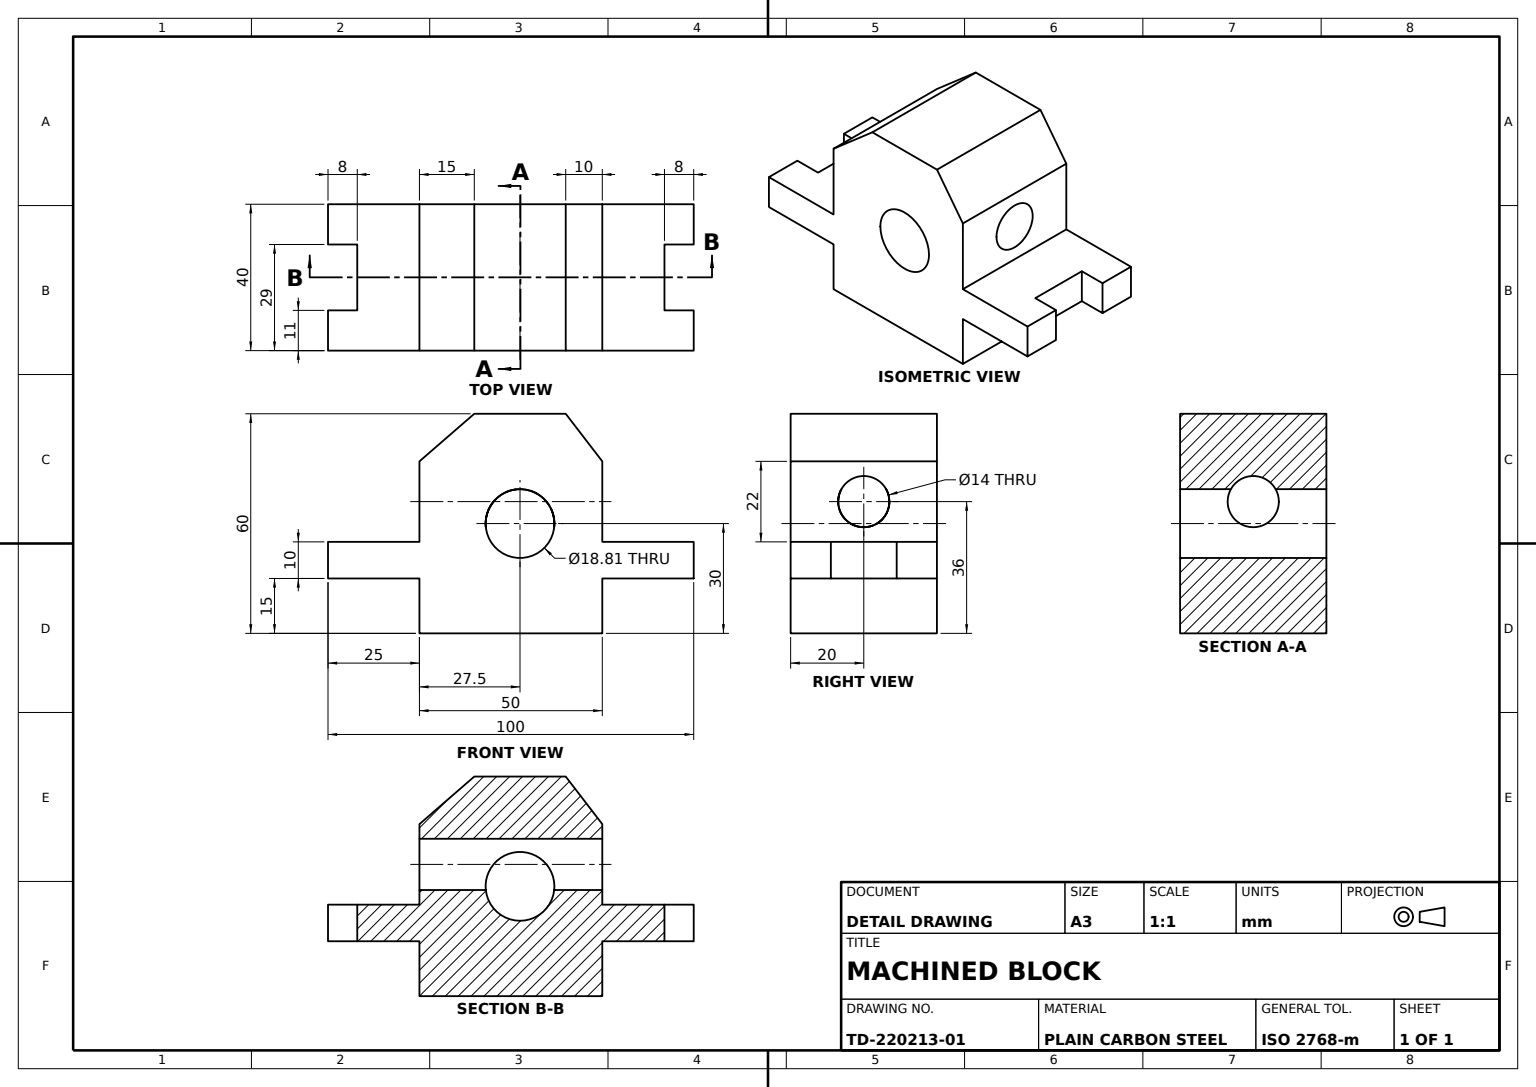
from build123d import *

# Parameters (mm, degrees)
BRACKET_BODY_DEPTH      = 40
FRONT_BORE_SKETCH_R     = 9.403768256
FRONT_BORE_DEPTH        = 105.043260233
FLANGE_NOTCH_SKETCH_W   = 8
FLANGE_NOTCH_SKETCH_H   = 18
FLANGE_NOTCH_CUTS_DEPTH = 40
FLANGE_SLOT_SKETCH_W    = 8
FLANGE_SLOT_SKETCH_H    = 18
FLANGE_SLOT_CUT_DEPTH   = 40
CROSS_HOLE_SKETCH_R     = 7
CROSS_HOLE_14_DEPTH     = 105.043260233


with BuildPart() as part:
    # Bracket Profile Sketch → Bracket Body (new body)
    with BuildSketch(Plane.XY):
        Polygon((0, 0), (50, 0), (50, 15), (75, 15), (75, 25), (50, 25), (50, 47), (40, 60), (15, 60), (0, 47), (0, 25), (-25, 25), (-25, 15), (0, 15), align=None)
    extrude(amount=BRACKET_BODY_DEPTH)

    # Front Bore Sketch → Front Bore (cut, through all)
    with BuildSketch(Plane.XY.offset(40)):
        with Locations((27.5, 30)):
            Circle(FRONT_BORE_SKETCH_R)
    extrude(amount=-FRONT_BORE_DEPTH, mode=Mode.SUBTRACT)

    # Flange Notch Sketch → Flange Notch Cuts (cut)
    with BuildSketch(Plane(origin=(0, 25, 0), x_dir=(1, 0, 0), z_dir=(0, 1, 0))):
        with Locations((71, -20)):
            Rectangle(FLANGE_NOTCH_SKETCH_W, FLANGE_NOTCH_SKETCH_H)
    extrude(amount=-FLANGE_NOTCH_CUTS_DEPTH, mode=Mode.SUBTRACT)

    # Flange Slot Sketch → Flange Slot Cut (cut)
    with BuildSketch(Plane(origin=(0, 25, 0), x_dir=(1, 0, 0), z_dir=(0, 1, 0))):
        with Locations((-21, -20)):
            Rectangle(FLANGE_SLOT_SKETCH_W, FLANGE_SLOT_SKETCH_H)
    extrude(amount=-FLANGE_SLOT_CUT_DEPTH, mode=Mode.SUBTRACT)

    # Cross Hole Sketch → Cross Hole Ø14 (cut, through all)
    with BuildSketch(Plane(origin=(50, 0, 0), x_dir=(0, 0, -1), z_dir=(1, 0, 0))):
        with Locations((-20, 36)):
            Circle(CROSS_HOLE_SKETCH_R)
    extrude(amount=-CROSS_HOLE_14_DEPTH, mode=Mode.SUBTRACT)


solid = part.part
